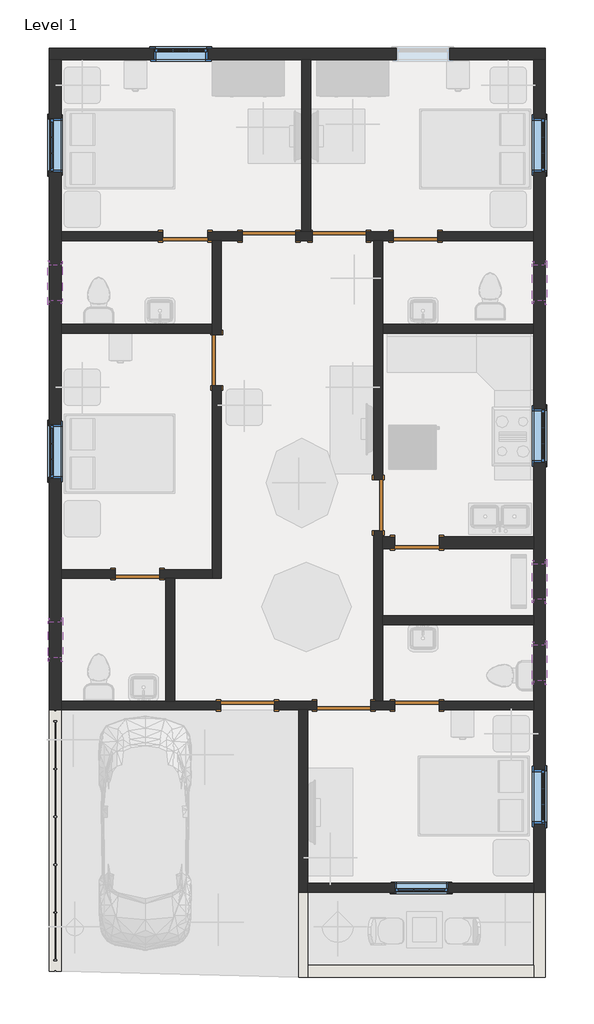
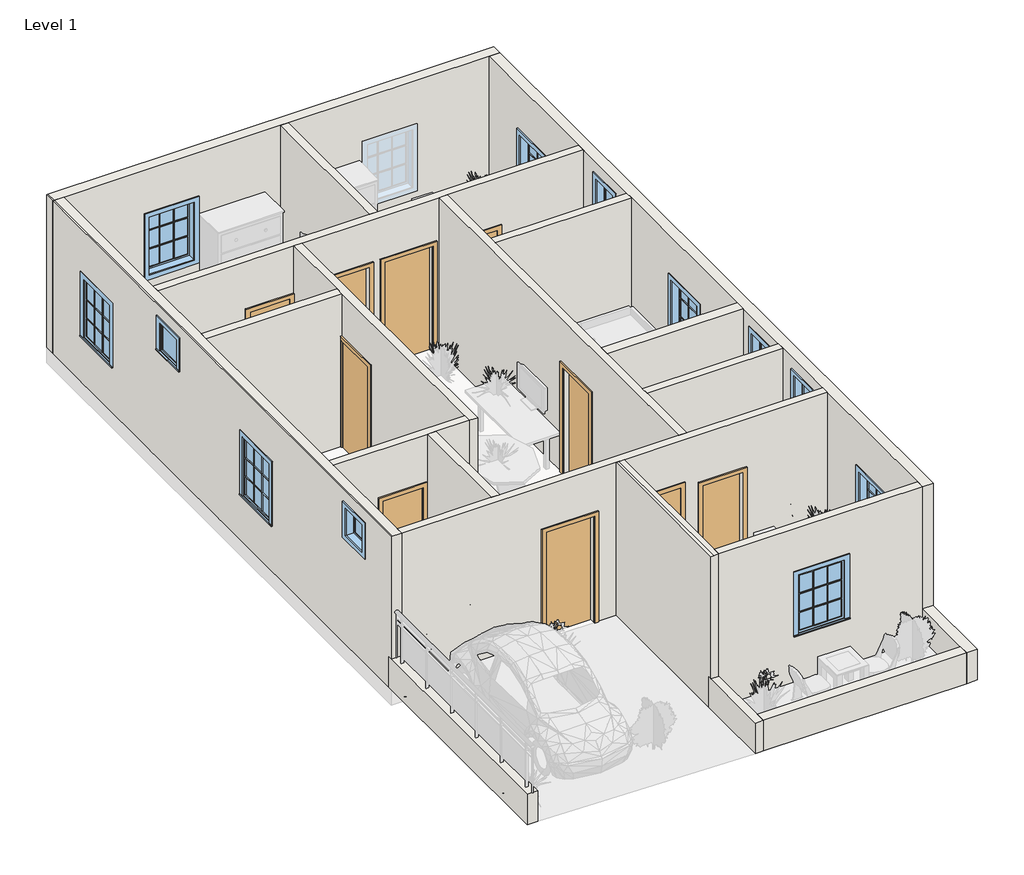
# One storey, part 1 of 2: 20 walls, 12 windows, 11 doors.
"""IFC4 building model written with IfcOpenShell, lengths in millimetres."""

from ifc_helpers import new_model, si_unit, frame, origin, origin_with_axes, place, context, project, spatial, polyline, outline, extrude, faceted_brep, transform, mapped, element, save
from components import door_255cab33, door_059fdd7e, door_fadea3f2, door_b6e9fca3, door_16372e1c, door_686f89d2, window_29c06734, window_5c190c7e, window_e41d21a6

model = new_model("IFC4")

# Units and contexts
model_context = context("Model", 3, world=origin())
ifc_project = project(units=[si_unit("LENGTHUNIT", "METRE", prefix="MILLI")], contexts=[model_context])

# Site, building, storey
site = spatial("IfcSite", under=ifc_project)
building = spatial("IfcBuilding", under=site)
storey = spatial("IfcBuildingStorey", under=building, Name="Level 1", Elevation=0.0)

# Doors
placement = place(None, origin())
door_shape = door_255cab33(model_context)
element("IfcDoor", 1, ObjectType="Single-Flush : 30\" x 80\"", at=placement, inside=storey, context=model_context, shape_type="MappedRepresentation", body=[
    mapped(door_shape, transform((-14104.3267032, 10209.9187882, 0.0), x_axis=(1.0, 0.0, 0.0), y_axis=(0.0, 1.0, 0.0), z_axis=(0.0, 0.0, 1.0))),
])
element("IfcDoor", 2, ObjectType="Single-Flush : 30\" x 80\"", at=placement, inside=storey, context=model_context, shape_type="MappedRepresentation", body=[
    mapped(door_shape, transform((-10167.3267032, 2234.3187882, 0.0), x_axis=(-1.0, 0.0, 0.0), y_axis=(0.0, -1.0, 0.0), z_axis=(0.0, 0.0, 1.0))),
])
element("IfcDoor", 3, ObjectType="Single-Flush : 30\" x 80\"", at=placement, inside=storey, context=model_context, shape_type="MappedRepresentation", body=[
    mapped(door_shape, transform((-14917.1267032, 4469.5187882, 0.0), x_axis=(1.0, 0.0, 0.0), y_axis=(0.0, 1.0, 0.0), z_axis=(0.0, 0.0, 1.0))),
])
door_2_shape = door_059fdd7e(model_context)
element("IfcDoor", 4, ObjectType="Single-Flush : 30\" x 80\"", at=placement, inside=storey, context=model_context, shape_type="MappedRepresentation", body=[
    mapped(door_2_shape, transform((-10192.7267032, 10209.9187882, 0.0), x_axis=(-1.0, 0.0, 0.0), y_axis=(0.0, -1.0, 0.0), z_axis=(0.0, 0.0, 1.0))),
])
door_3_shape = door_fadea3f2(model_context)
element("IfcDoor", 5, ObjectType="Single-Flush : 30\" x 80\"", at=placement, inside=storey, context=model_context, shape_type="MappedRepresentation", body=[
    mapped(door_3_shape, transform((-10167.3267032, 5002.9187882, 0.0), x_axis=(-1.0, 0.0, 0.0), y_axis=(0.0, -1.0, 0.0), z_axis=(0.0, 0.0, 1.0))),
])
door_4_shape = door_b6e9fca3(model_context)
element("IfcDoor", 6, ObjectType="Single-Flush : 34\" x 84\"", at=placement, inside=storey, context=model_context, shape_type="MappedRepresentation", body=[
    mapped(door_4_shape, transform((-13570.9267032, 8101.7187882, 0.0), x_axis=(0.0, 1.0, 0.0), y_axis=(-1.0, 0.0, 0.0), z_axis=(0.0, 0.0, 1.0))),
])
element("IfcDoor", 7, ObjectType="Single-Flush : 34\" x 84\"", at=placement, inside=storey, context=model_context, shape_type="MappedRepresentation", body=[
    mapped(door_4_shape, transform((-10827.7267032, 5637.9187882, 0.0), x_axis=(0.0, -1.0, 0.0), y_axis=(1.0, 0.0, 0.0), z_axis=(0.0, 0.0, 1.0))),
])
door_5_shape = door_16372e1c(model_context)
element("IfcDoor", 8, ObjectType="Single-Flush : 36\" x 84\"", at=placement, inside=storey, context=model_context, shape_type="MappedRepresentation", body=[
    mapped(door_5_shape, transform((-12681.9267032, 10209.9187882, 0.0), x_axis=(1.0, 0.0, 0.0), y_axis=(0.0, 1.0, 0.0), z_axis=(0.0, 0.0, 1.0))),
])
element("IfcDoor", 9, ObjectType="Single-Flush : 36\" x 84\"", at=placement, inside=storey, context=model_context, shape_type="MappedRepresentation", body=[
    mapped(door_5_shape, transform((-11411.9267032, 2234.3187882, 0.0), x_axis=(-1.0, 0.0, 0.0), y_axis=(0.0, -1.0, 0.0), z_axis=(0.0, 0.0, 1.0))),
])
door_6_shape = door_686f89d2(model_context)
element("IfcDoor", 10, ObjectType="Single-Flush : 36\" x 84\"", at=placement, inside=storey, context=model_context, shape_type="MappedRepresentation", body=[
    mapped(door_6_shape, transform((-11488.1267032, 10209.9187882, 0.0), x_axis=(-1.0, 0.0, 0.0), y_axis=(0.0, -1.0, 0.0), z_axis=(0.0, 0.0, 1.0))),
])
element("IfcDoor", 11, ObjectType="Single-Flush : 36\" x 84\"", at=placement, inside=storey, context=model_context, shape_type="MappedRepresentation", body=[
    mapped(door_6_shape, transform((-13050.2267032, 2234.3187882, 0.0), x_axis=(-1.0, 0.0, 0.0), y_axis=(0.0, -1.0, 0.0), z_axis=(0.0, 0.0, 1.0))),
])

# Walls
element("IfcWall", 12, ObjectType="Generic - 2'", at=placement, inside=storey, context=model_context, shape_type="Brep", body=[
    faceted_brep([(-16212.5267032, -2286.8812118, 0.0), (-16212.5267032, 2158.1187882, 0.0), (-16212.5267032, 2234.3187882, 0.0), (-16212.5267032, 2234.3187882, 609.6), (-16212.5267032, -2286.8812118, 609.6), (-16415.7267032, -2286.8812118, 0.0), (-16415.7267032, -2286.8812118, 609.6), (-16415.7267032, 2234.3187882, 609.6), (-16415.7267032, 2234.3187882, 0.0)], [[[0, 1, 2, 3, 4]], [[5, 6, 7, 8]], [[2, 1, 0, 5, 8]], [[3, 2, 8, 7]], [[4, 3, 7, 6]], [[0, 4, 6, 5]]]),
])
element("IfcWall", 13, ObjectType="Generic - 2'", at=placement, inside=storey, context=model_context, shape_type="SweptSolid", body=[
    extrude(outline(polyline([(-12021.5267032, -2185.2812118), (-8186.1267032, -2185.2812118), (-8186.1267032, -2388.4812118), (-12021.5267032, -2388.4812118), (-12021.5267032, -2185.2812118)])), origin_with_axes(), (0.0, 0.0, 1.0), 609.6),
])
element("IfcWall", 14, ObjectType="Generic - 2'", at=placement, inside=storey, context=model_context, shape_type="Brep", body=[
    faceted_brep([(-8186.1267032, -864.4812118, 0.0), (-8186.1267032, -940.6812118, 0.0), (-8186.1267032, -2185.2812118, 0.0), (-8186.1267032, -2388.4812118, 0.0), (-8186.1267032, -2388.4812118, 609.6), (-8186.1267032, -2185.2812118, 609.6), (-8186.1267032, -864.4812118, 609.6), (-7982.9267032, -864.4812118, 0.0), (-7982.9267032, -864.4812118, 609.6), (-7982.9267032, -2388.4812118, 609.6), (-7982.9267032, -2388.4812118, 0.0)], [[[0, 1, 2, 3, 4, 5, 6]], [[7, 8, 9, 10]], [[3, 2, 1, 0, 7, 10]], [[6, 5, 4, 9, 8]], [[0, 6, 8, 7]], [[4, 3, 10, 9]]]),
])
element("IfcWall", 15, ObjectType="Generic - 8\"", at=placement, inside=storey, context=model_context, shape_type="Brep", body=[
    faceted_brep([(-16415.7267032, 13207.1187882, 0.0), (-16212.5267032, 13207.1187882, 0.0), (-12123.1267032, 13207.1187882, 0.0), (-11970.7267032, 13207.1187882, 0.0), (-8186.1267032, 13207.1187882, 0.0), (-7982.9267032, 13207.1187882, 0.0), (-7982.9267032, 13207.1187882, 3048.0), (-8186.1267032, 13207.1187882, 3048.0), (-11970.7267032, 13207.1187882, 3048.0), (-12123.1267032, 13207.1187882, 3048.0), (-16212.5267032, 13207.1187882, 3048.0), (-16390.3267032, 13207.1187882, 3048.0), (-16415.7267032, 13207.1187882, 3048.0), (-13723.3267032, 13207.1187882, 2133.6), (-13723.3267032, 13207.1187882, 914.4), (-14637.7267032, 13207.1187882, 914.4), (-14637.7267032, 13207.1187882, 2133.6), (-9608.5267032, 13207.1187882, 2133.6), (-9608.5267032, 13207.1187882, 914.4), (-10522.9267032, 13207.1187882, 914.4), (-10522.9267032, 13207.1187882, 2133.6), (-16415.7267032, 13410.3187882, 0.0), (-16415.7267032, 13410.3187882, 3048.0), (-16390.3267032, 13410.3187882, 3048.0), (-7982.9267032, 13410.3187882, 3048.0), (-7982.9267032, 13410.3187882, 0.0), (-13723.3267032, 13410.3187882, 2133.6), (-14637.7267032, 13410.3187882, 2133.6), (-14637.7267032, 13410.3187882, 914.4), (-13723.3267032, 13410.3187882, 914.4), (-9608.5267032, 13410.3187882, 2133.6), (-10522.9267032, 13410.3187882, 2133.6), (-10522.9267032, 13410.3187882, 914.4), (-9608.5267032, 13410.3187882, 914.4)], [[[0, 1, 2, 3, 4, 5, 6, 7, 8, 9, 10, 11, 12], [13, 14, 15, 16], [17, 18, 19, 20]], [[21, 22, 23, 24, 25], [26, 27, 28, 29], [30, 31, 32, 33]], [[5, 4, 3, 2, 1, 0, 21, 25]], [[6, 5, 25, 24]], [[0, 12, 22, 21]], [[14, 13, 26, 29]], [[15, 14, 29, 28]], [[16, 15, 28, 27]], [[13, 16, 27, 26]], [[18, 17, 30, 33]], [[19, 18, 33, 32]], [[20, 19, 32, 31]], [[17, 20, 31, 30]], [[12, 11, 23, 22]], [[11, 10, 9, 8, 7, 6, 24, 23]]]),
])
element("IfcWall", 16, ObjectType="Generic - 8\"", at=placement, inside=storey, context=model_context, shape_type="Brep", body=[
    faceted_brep([(-8186.1267032, 13207.1187882, 0.0), (-8186.1267032, 10286.1187882, 0.0), (-8186.1267032, 10133.7187882, 0.0), (-8186.1267032, 8711.3187882, 0.0), (-8186.1267032, 8558.9187882, 0.0), (-8186.1267032, 5104.5187882, 0.0), (-8186.1267032, 4901.3187882, 0.0), (-8186.1267032, 3758.3187882, 0.0), (-8186.1267032, 3605.9187882, 0.0), (-8186.1267032, 2310.5187882, 0.0), (-8186.1267032, 2158.1187882, 0.0), (-8186.1267032, -788.2812118, 0.0), (-8186.1267032, -864.4812118, 0.0), (-8186.1267032, -864.4812118, 609.6), (-8186.1267032, -940.6812118, 609.6), (-8186.1267032, -940.6812118, 3048.0), (-8186.1267032, -788.2812118, 3048.0), (-8186.1267032, 2158.1187882, 3048.0), (-8186.1267032, 2310.5187882, 3048.0), (-8186.1267032, 3605.9187882, 3048.0), (-8186.1267032, 3758.3187882, 3048.0), (-8186.1267032, 4901.3187882, 3048.0), (-8186.1267032, 5104.5187882, 3048.0), (-8186.1267032, 8558.9187882, 3048.0), (-8186.1267032, 8711.3187882, 3048.0), (-8186.1267032, 10133.7187882, 3048.0), (-8186.1267032, 10286.1187882, 3048.0), (-8186.1267032, 13207.1187882, 3048.0), (-8186.1267032, 11302.1187882, 2133.6), (-8186.1267032, 11302.1187882, 914.4), (-8186.1267032, 12216.5187882, 914.4), (-8186.1267032, 12216.5187882, 2133.6), (-8186.1267032, 6361.8187882, 2235.2), (-8186.1267032, 6361.8187882, 1016.0), (-8186.1267032, 7276.2187882, 1016.0), (-8186.1267032, 7276.2187882, 2235.2), (-8186.1267032, 227.7187882, 2133.6), (-8186.1267032, 227.7187882, 914.4), (-8186.1267032, 1142.1187882, 914.4), (-8186.1267032, 1142.1187882, 2133.6), (-8186.1267032, 4037.7187882, 2768.6), (-8186.1267032, 4037.7187882, 2159.0), (-8186.1267032, 4647.3187882, 2159.0), (-8186.1267032, 4647.3187882, 2768.6), (-8186.1267032, 2653.4187882, 2768.6), (-8186.1267032, 2653.4187882, 2159.0), (-8186.1267032, 3263.0187882, 2159.0), (-8186.1267032, 3263.0187882, 2768.6), (-8186.1267032, 9117.7187882, 2768.6), (-8186.1267032, 9117.7187882, 2159.0), (-8186.1267032, 9727.3187882, 2159.0), (-8186.1267032, 9727.3187882, 2768.6), (-7982.9267032, 13207.1187882, 0.0), (-7982.9267032, 13207.1187882, 3048.0), (-7982.9267032, -940.6812118, 3048.0), (-7982.9267032, -940.6812118, 609.6), (-7982.9267032, -864.4812118, 609.6), (-7982.9267032, -864.4812118, 0.0), (-7982.9267032, 11302.1187882, 2133.6), (-7982.9267032, 12216.5187882, 2133.6), (-7982.9267032, 12216.5187882, 914.4), (-7982.9267032, 11302.1187882, 914.4), (-7982.9267032, 6361.8187882, 2235.2), (-7982.9267032, 7276.2187882, 2235.2), (-7982.9267032, 7276.2187882, 1016.0), (-7982.9267032, 6361.8187882, 1016.0), (-7982.9267032, 227.7187882, 2133.6), (-7982.9267032, 1142.1187882, 2133.6), (-7982.9267032, 1142.1187882, 914.4), (-7982.9267032, 227.7187882, 914.4), (-7982.9267032, 4037.7187882, 2768.6), (-7982.9267032, 4647.3187882, 2768.6), (-7982.9267032, 4647.3187882, 2159.0), (-7982.9267032, 4037.7187882, 2159.0), (-7982.9267032, 2653.4187882, 2768.6), (-7982.9267032, 3263.0187882, 2768.6), (-7982.9267032, 3263.0187882, 2159.0), (-7982.9267032, 2653.4187882, 2159.0), (-7982.9267032, 9117.7187882, 2768.6), (-7982.9267032, 9727.3187882, 2768.6), (-7982.9267032, 9727.3187882, 2159.0), (-7982.9267032, 9117.7187882, 2159.0)], [[[0, 1, 2, 3, 4, 5, 6, 7, 8, 9, 10, 11, 12, 13, 14, 15, 16, 17, 18, 19, 20, 21, 22, 23, 24, 25, 26, 27], [28, 29, 30, 31], [32, 33, 34, 35], [36, 37, 38, 39], [40, 41, 42, 43], [44, 45, 46, 47], [48, 49, 50, 51]], [[52, 53, 54, 55, 56, 57], [58, 59, 60, 61], [62, 63, 64, 65], [66, 67, 68, 69], [70, 71, 72, 73], [74, 75, 76, 77], [78, 79, 80, 81]], [[12, 11, 10, 9, 8, 7, 6, 5, 4, 3, 2, 1, 0, 52, 57]], [[0, 27, 53, 52]], [[29, 28, 58, 61]], [[30, 29, 61, 60]], [[31, 30, 60, 59]], [[28, 31, 59, 58]], [[33, 32, 62, 65]], [[34, 33, 65, 64]], [[35, 34, 64, 63]], [[32, 35, 63, 62]], [[37, 36, 66, 69]], [[38, 37, 69, 68]], [[39, 38, 68, 67]], [[36, 39, 67, 66]], [[41, 40, 70, 73]], [[42, 41, 73, 72]], [[43, 42, 72, 71]], [[40, 43, 71, 70]], [[45, 44, 74, 77]], [[46, 45, 77, 76]], [[47, 46, 76, 75]], [[44, 47, 75, 74]], [[49, 48, 78, 81]], [[50, 49, 81, 80]], [[51, 50, 80, 79]], [[48, 51, 79, 78]], [[13, 12, 57, 56]], [[55, 14, 13, 56]], [[15, 14, 55, 54]], [[27, 26, 25, 24, 23, 22, 21, 20, 19, 18, 17, 16, 15, 54, 53]]]),
])
element("IfcWall", 17, ObjectType="Generic - 8\"", at=placement, inside=storey, context=model_context, shape_type="SweptSolid", body=[
    extrude(outline(polyline([(0.0, -10751.5267032), (0.0, -10548.3267032), (2032.0, -10548.3267032), (2032.0, -9786.3267032), (0.0, -9786.3267032), (0.0, -8186.1267032), (3048.0, -8186.1267032), (3048.0, -10751.5267032), (0.0, -10751.5267032)])), frame((0.0, 4901.3187882, 0.0), z_axis=(0.0, 1.0, 0.0), x_axis=(0.0, 0.0, 1.0)), (0.0, 0.0, 1.0), 203.2),
])
element("IfcWall", 18, ObjectType="Generic - 8\"", at=placement, inside=storey, context=model_context, shape_type="Brep", body=[
    faceted_brep([(-16212.5267032, 2234.3187882, 0.0), (-16212.5267032, 2310.5187882, 0.0), (-16212.5267032, 4393.3187882, 0.0), (-16212.5267032, 4545.7187882, 0.0), (-16212.5267032, 8558.9187882, 0.0), (-16212.5267032, 8711.3187882, 0.0), (-16212.5267032, 10133.7187882, 0.0), (-16212.5267032, 10286.1187882, 0.0), (-16212.5267032, 13207.1187882, 0.0), (-16212.5267032, 13207.1187882, 3048.0), (-16212.5267032, 10286.1187882, 3048.0), (-16212.5267032, 10133.7187882, 3048.0), (-16212.5267032, 8711.3187882, 3048.0), (-16212.5267032, 8558.9187882, 3048.0), (-16212.5267032, 4545.7187882, 3048.0), (-16212.5267032, 4393.3187882, 3048.0), (-16212.5267032, 2310.5187882, 3048.0), (-16212.5267032, 2158.1187882, 3048.0), (-16212.5267032, 2158.1187882, 609.6), (-16212.5267032, 2234.3187882, 609.6), (-16212.5267032, 12216.5187882, 2133.6), (-16212.5267032, 12216.5187882, 914.4), (-16212.5267032, 11302.1187882, 914.4), (-16212.5267032, 11302.1187882, 2133.6), (-16212.5267032, 7009.5187882, 2133.6), (-16212.5267032, 7009.5187882, 914.4), (-16212.5267032, 6095.1187882, 914.4), (-16212.5267032, 6095.1187882, 2133.6), (-16212.5267032, 3047.1187882, 2768.6), (-16212.5267032, 3656.7187882, 2768.6), (-16212.5267032, 3656.7187882, 2159.0), (-16212.5267032, 3047.1187882, 2159.0), (-16212.5267032, 9727.3187882, 2768.6), (-16212.5267032, 9727.3187882, 2159.0), (-16212.5267032, 9117.7187882, 2159.0), (-16212.5267032, 9117.7187882, 2768.6), (-16415.7267032, 2234.3187882, 0.0), (-16415.7267032, 2234.3187882, 609.6), (-16415.7267032, 2158.1187882, 609.6), (-16415.7267032, 2158.1187882, 3048.0), (-16415.7267032, 13207.1187882, 3048.0), (-16415.7267032, 13207.1187882, 0.0), (-16415.7267032, 12216.5187882, 2133.6), (-16415.7267032, 11302.1187882, 2133.6), (-16415.7267032, 11302.1187882, 914.4), (-16415.7267032, 12216.5187882, 914.4), (-16415.7267032, 7009.5187882, 2133.6), (-16415.7267032, 6095.1187882, 2133.6), (-16415.7267032, 6095.1187882, 914.4), (-16415.7267032, 7009.5187882, 914.4), (-16415.7267032, 3047.1187882, 2768.6), (-16415.7267032, 3047.1187882, 2159.0), (-16415.7267032, 3656.7187882, 2159.0), (-16415.7267032, 3656.7187882, 2768.6), (-16415.7267032, 9727.3187882, 2768.6), (-16415.7267032, 9117.7187882, 2768.6), (-16415.7267032, 9117.7187882, 2159.0), (-16415.7267032, 9727.3187882, 2159.0), (-16390.3267032, 13207.1187882, 3048.0), (-16390.3267032, 2158.1187882, 3048.0)], [[[0, 1, 2, 3, 4, 5, 6, 7, 8, 9, 10, 11, 12, 13, 14, 15, 16, 17, 18, 19], [20, 21, 22, 23], [24, 25, 26, 27], [28, 29, 30, 31], [32, 33, 34, 35]], [[36, 37, 38, 39, 40, 41], [42, 43, 44, 45], [46, 47, 48, 49], [50, 51, 52, 53], [54, 55, 56, 57]], [[8, 7, 6, 5, 4, 3, 2, 1, 0, 36, 41]], [[9, 8, 41, 40, 58]], [[20, 23, 43, 42]], [[23, 22, 44, 43]], [[22, 21, 45, 44]], [[21, 20, 42, 45]], [[24, 27, 47, 46]], [[27, 26, 48, 47]], [[26, 25, 49, 48]], [[25, 24, 46, 49]], [[50, 53, 29, 28]], [[53, 52, 30, 29]], [[52, 51, 31, 30]], [[51, 50, 28, 31]], [[32, 35, 55, 54]], [[35, 34, 56, 55]], [[34, 33, 57, 56]], [[33, 32, 54, 57]], [[0, 19, 37, 36]], [[18, 38, 37, 19]], [[18, 17, 59, 39, 38]], [[58, 40, 39, 59]], [[17, 16, 15, 14, 13, 12, 11, 10, 9, 58, 59]]]),
])
element("IfcWall", 19, ObjectType="INNER 6\"", at=placement, inside=storey, context=model_context, shape_type="SweptSolid", body=[
    extrude(outline(polyline([(-12123.1267032, 10286.1187882), (-12123.1267032, 13207.1187882), (-11970.7267032, 13207.1187882), (-11970.7267032, 10286.1187882), (-12123.1267032, 10286.1187882)])), origin_with_axes(), (0.0, 0.0, 1.0), 3048.0),
])
element("IfcWall", 20, ObjectType="INNER 6\"", at=placement, inside=storey, context=model_context, shape_type="Brep", body=[
    faceted_brep([(-10573.7267032, 10286.1187882, 2032.0), (-10573.7267032, 10286.1187882, 0.0), (-11030.9267032, 10286.1187882, 0.0), (-11030.9267032, 10286.1187882, 2133.6), (-11945.3267032, 10286.1187882, 2133.6), (-11945.3267032, 10286.1187882, 0.0), (-11970.7267032, 10286.1187882, 0.0), (-12123.1267032, 10286.1187882, 0.0), (-12224.7267032, 10286.1187882, 0.0), (-12224.7267032, 10286.1187882, 2133.6), (-13139.1267032, 10286.1187882, 2133.6), (-13139.1267032, 10286.1187882, 0.0), (-13723.3267032, 10286.1187882, 0.0), (-13723.3267032, 10286.1187882, 2032.0), (-14485.3267032, 10286.1187882, 2032.0), (-14485.3267032, 10286.1187882, 0.0), (-16212.5267032, 10286.1187882, 0.0), (-16212.5267032, 10286.1187882, 3048.0), (-12123.1267032, 10286.1187882, 3048.0), (-11970.7267032, 10286.1187882, 3048.0), (-8186.1267032, 10286.1187882, 3048.0), (-8186.1267032, 10286.1187882, 0.0), (-9811.7267032, 10286.1187882, 0.0), (-9811.7267032, 10286.1187882, 2032.0), (-11030.9267032, 10133.7187882, 0.0), (-10903.9267032, 10133.7187882, 0.0), (-10751.5267032, 10133.7187882, 0.0), (-10573.7267032, 10133.7187882, 0.0), (-10573.7267032, 10133.7187882, 2032.0), (-9811.7267032, 10133.7187882, 2032.0), (-9811.7267032, 10133.7187882, 0.0), (-8186.1267032, 10133.7187882, 0.0), (-8186.1267032, 10133.7187882, 3048.0), (-10751.5267032, 10133.7187882, 3048.0), (-10903.9267032, 10133.7187882, 3048.0), (-13494.7267032, 10133.7187882, 3048.0), (-13647.1267032, 10133.7187882, 3048.0), (-16212.5267032, 10133.7187882, 3048.0), (-16212.5267032, 10133.7187882, 0.0), (-14485.3267032, 10133.7187882, 0.0), (-14485.3267032, 10133.7187882, 2032.0), (-13723.3267032, 10133.7187882, 2032.0), (-13723.3267032, 10133.7187882, 0.0), (-13647.1267032, 10133.7187882, 0.0), (-13494.7267032, 10133.7187882, 0.0), (-13139.1267032, 10133.7187882, 0.0), (-13139.1267032, 10133.7187882, 2133.6), (-12224.7267032, 10133.7187882, 2133.6), (-12224.7267032, 10133.7187882, 0.0), (-11945.3267032, 10133.7187882, 0.0), (-11945.3267032, 10133.7187882, 2133.6), (-11030.9267032, 10133.7187882, 2133.6)], [[[0, 1, 2, 3, 4, 5, 6, 7, 8, 9, 10, 11, 12, 13, 14, 15, 16, 17, 18, 19, 20, 21, 22, 23]], [[24, 25, 26, 27, 28, 29, 30, 31, 32, 33, 34, 35, 36, 37, 38, 39, 40, 41, 42, 43, 44, 45, 46, 47, 48, 49, 50, 51]], [[8, 7, 6, 5, 49, 48]], [[39, 38, 16, 15]], [[45, 44, 43, 42, 12, 11]], [[22, 21, 31, 30]], [[2, 1, 27, 26, 25, 24]], [[17, 16, 38, 37]], [[21, 20, 32, 31]], [[9, 8, 48, 47]], [[10, 9, 47, 46]], [[11, 10, 46, 45]], [[50, 49, 5, 4]], [[51, 50, 4, 3]], [[24, 51, 3, 2]], [[13, 12, 42, 41]], [[14, 13, 41, 40]], [[15, 14, 40, 39]], [[28, 27, 1, 0]], [[29, 28, 0, 23]], [[30, 29, 23, 22]], [[20, 19, 18, 17, 37, 36, 35, 34, 33, 32]]]),
])
element("IfcWall", 21, ObjectType="INNER 6\"", at=placement, inside=storey, context=model_context, shape_type="Brep", body=[
    faceted_brep([(-13647.1267032, 10133.7187882, 0.0), (-13647.1267032, 8711.3187882, 0.0), (-13647.1267032, 8558.9187882, 0.0), (-13647.1267032, 8533.5187882, 0.0), (-13647.1267032, 8533.5187882, 2133.6), (-13647.1267032, 7669.9187882, 2133.6), (-13647.1267032, 7669.9187882, 0.0), (-13647.1267032, 4545.7187882, 0.0), (-13647.1267032, 4393.3187882, 0.0), (-13647.1267032, 4393.3187882, 3048.0), (-13647.1267032, 4545.7187882, 3048.0), (-13647.1267032, 8558.9187882, 3048.0), (-13647.1267032, 8711.3187882, 3048.0), (-13647.1267032, 10133.7187882, 3048.0), (-13494.7267032, 8533.5187882, 2133.6), (-13494.7267032, 8533.5187882, 0.0), (-13494.7267032, 10133.7187882, 0.0), (-13494.7267032, 10133.7187882, 3048.0), (-13494.7267032, 4393.3187882, 3048.0), (-13494.7267032, 4393.3187882, 0.0), (-13494.7267032, 7669.9187882, 0.0), (-13494.7267032, 7669.9187882, 2133.6)], [[[0, 1, 2, 3, 4, 5, 6, 7, 8, 9, 10, 11, 12, 13]], [[14, 15, 16, 17, 18, 19, 20, 21]], [[20, 19, 8, 7, 6]], [[16, 15, 3, 2, 1, 0]], [[0, 13, 17, 16]], [[9, 8, 19, 18]], [[4, 3, 15, 14]], [[5, 4, 14, 21]], [[6, 5, 21, 20]], [[13, 12, 11, 10, 9, 18, 17]]]),
])
element("IfcWall", 22, ObjectType="INNER 6\"", at=placement, inside=storey, context=model_context, shape_type="SweptSolid", body=[
    extrude(outline(polyline([(-16212.5267032, 8711.3187882), (-13647.1267032, 8711.3187882), (-13647.1267032, 8558.9187882), (-16212.5267032, 8558.9187882), (-16212.5267032, 8711.3187882)])), origin_with_axes(), (0.0, 0.0, 1.0), 3048.0),
])
element("IfcWall", 23, ObjectType="INNER 6\"", at=placement, inside=storey, context=model_context, shape_type="SweptSolid", body=[
    extrude(outline(polyline([(-8186.1267032, 8558.9187882), (-10751.5267032, 8558.9187882), (-10751.5267032, 8711.3187882), (-8186.1267032, 8711.3187882), (-8186.1267032, 8558.9187882)])), origin_with_axes(), (0.0, 0.0, 1.0), 3048.0),
])
element("IfcWall", 24, ObjectType="INNER 6\"", at=placement, inside=storey, context=model_context, shape_type="Brep", body=[
    faceted_brep([(-10903.9267032, 5206.1187882, 2133.6), (-10903.9267032, 5206.1187882, 0.0), (-10903.9267032, 2310.5187882, 0.0), (-10903.9267032, 2310.5187882, 3048.0), (-10903.9267032, 10133.7187882, 3048.0), (-10903.9267032, 10133.7187882, 0.0), (-10903.9267032, 6069.7187882, 0.0), (-10903.9267032, 6069.7187882, 2133.6), (-10751.5267032, 2310.5187882, 0.0), (-10751.5267032, 3605.9187882, 0.0), (-10751.5267032, 3758.3187882, 0.0), (-10751.5267032, 4901.3187882, 0.0), (-10751.5267032, 5104.5187882, 0.0), (-10751.5267032, 5206.1187882, 0.0), (-10751.5267032, 5206.1187882, 2133.6), (-10751.5267032, 6069.7187882, 2133.6), (-10751.5267032, 6069.7187882, 0.0), (-10751.5267032, 8558.9187882, 0.0), (-10751.5267032, 8711.3187882, 0.0), (-10751.5267032, 10133.7187882, 0.0), (-10751.5267032, 10133.7187882, 3048.0), (-10751.5267032, 8711.3187882, 3048.0), (-10751.5267032, 8558.9187882, 3048.0), (-10751.5267032, 5104.5187882, 3048.0), (-10751.5267032, 4901.3187882, 3048.0), (-10751.5267032, 3758.3187882, 3048.0), (-10751.5267032, 3605.9187882, 3048.0), (-10751.5267032, 2310.5187882, 3048.0)], [[[0, 1, 2, 3, 4, 5, 6, 7]], [[8, 9, 10, 11, 12, 13, 14, 15, 16, 17, 18, 19, 20, 21, 22, 23, 24, 25, 26, 27]], [[6, 5, 19, 18, 17, 16]], [[2, 1, 13, 12, 11, 10, 9, 8]], [[5, 4, 20, 19]], [[3, 2, 8, 27]], [[14, 13, 1, 0]], [[15, 14, 0, 7]], [[16, 15, 7, 6]], [[4, 3, 27, 26, 25, 24, 23, 22, 21, 20]]]),
])
element("IfcWall", 25, ObjectType="INNER 6\"", at=placement, inside=storey, context=model_context, shape_type="Brep", body=[
    faceted_brep([(-13647.1267032, 4545.7187882, 0.0), (-14536.1267032, 4545.7187882, 0.0), (-14536.1267032, 4545.7187882, 2032.0), (-15298.1267032, 4545.7187882, 2032.0), (-15298.1267032, 4545.7187882, 0.0), (-16212.5267032, 4545.7187882, 0.0), (-16212.5267032, 4545.7187882, 3048.0), (-13647.1267032, 4545.7187882, 3048.0), (-14536.1267032, 4393.3187882, 2032.0), (-14536.1267032, 4393.3187882, 0.0), (-14434.5267032, 4393.3187882, 0.0), (-14282.1267032, 4393.3187882, 0.0), (-13647.1267032, 4393.3187882, 0.0), (-13647.1267032, 4393.3187882, 3048.0), (-14282.1267032, 4393.3187882, 3048.0), (-14434.5267032, 4393.3187882, 3048.0), (-16212.5267032, 4393.3187882, 3048.0), (-16212.5267032, 4393.3187882, 0.0), (-15298.1267032, 4393.3187882, 0.0), (-15298.1267032, 4393.3187882, 2032.0)], [[[0, 1, 2, 3, 4, 5, 6, 7]], [[8, 9, 10, 11, 12, 13, 14, 15, 16, 17, 18, 19]], [[18, 17, 5, 4]], [[12, 11, 10, 9, 1, 0]], [[0, 7, 13, 12]], [[6, 5, 17, 16]], [[2, 1, 9, 8]], [[3, 2, 8, 19]], [[4, 3, 19, 18]], [[7, 6, 16, 15, 14, 13]]]),
])
element("IfcWall", 26, ObjectType="INNER 6\"", at=placement, inside=storey, context=model_context, shape_type="SweptSolid", body=[
    extrude(outline(polyline([(-14434.5267032, 2310.5187882), (-14434.5267032, 4393.3187882), (-14282.1267032, 4393.3187882), (-14282.1267032, 2310.5187882), (-14434.5267032, 2310.5187882)])), origin_with_axes(), (0.0, 0.0, 1.0), 3048.0),
])
element("IfcWall", 27, ObjectType="INNER 6\"", at=placement, inside=storey, context=model_context, shape_type="Brep", body=[
    faceted_brep([(-16212.5267032, 2158.1187882, 0.0), (-13507.4267032, 2158.1187882, 0.0), (-13507.4267032, 2158.1187882, 2133.6), (-12593.0267032, 2158.1187882, 2133.6), (-12593.0267032, 2158.1187882, 0.0), (-12173.9267032, 2158.1187882, 0.0), (-12021.5267032, 2158.1187882, 0.0), (-11869.1267032, 2158.1187882, 0.0), (-11869.1267032, 2158.1187882, 2133.6), (-10954.7267032, 2158.1187882, 2133.6), (-10954.7267032, 2158.1187882, 0.0), (-10548.3267032, 2158.1187882, 0.0), (-10548.3267032, 2158.1187882, 2032.0), (-9786.3267032, 2158.1187882, 2032.0), (-9786.3267032, 2158.1187882, 0.0), (-8186.1267032, 2158.1187882, 0.0), (-8186.1267032, 2158.1187882, 3048.0), (-12021.5267032, 2158.1187882, 3048.0), (-12173.9267032, 2158.1187882, 3048.0), (-16212.5267032, 2158.1187882, 3048.0), (-16212.5267032, 2158.1187882, 609.6), (-13507.4267032, 2310.5187882, 2133.6), (-13507.4267032, 2310.5187882, 0.0), (-14282.1267032, 2310.5187882, 0.0), (-14434.5267032, 2310.5187882, 0.0), (-16212.5267032, 2310.5187882, 0.0), (-16212.5267032, 2310.5187882, 3048.0), (-14434.5267032, 2310.5187882, 3048.0), (-14282.1267032, 2310.5187882, 3048.0), (-10903.9267032, 2310.5187882, 3048.0), (-10751.5267032, 2310.5187882, 3048.0), (-8186.1267032, 2310.5187882, 3048.0), (-8186.1267032, 2310.5187882, 0.0), (-9786.3267032, 2310.5187882, 0.0), (-9786.3267032, 2310.5187882, 2032.0), (-10548.3267032, 2310.5187882, 2032.0), (-10548.3267032, 2310.5187882, 0.0), (-10751.5267032, 2310.5187882, 0.0), (-10903.9267032, 2310.5187882, 0.0), (-10954.7267032, 2310.5187882, 0.0), (-10954.7267032, 2310.5187882, 2133.6), (-11869.1267032, 2310.5187882, 2133.6), (-11869.1267032, 2310.5187882, 0.0), (-12593.0267032, 2310.5187882, 0.0), (-12593.0267032, 2310.5187882, 2133.6), (-16212.5267032, 2234.3187882, 0.0)], [[[0, 1, 2, 3, 4, 5, 6, 7, 8, 9, 10, 11, 12, 13, 14, 15, 16, 17, 18, 19, 20]], [[21, 22, 23, 24, 25, 26, 27, 28, 29, 30, 31, 32, 33, 34, 35, 36, 37, 38, 39, 40, 41, 42, 43, 44]], [[33, 32, 15, 14]], [[39, 38, 37, 36, 11, 10]], [[43, 42, 7, 6, 5, 4]], [[25, 24, 23, 22, 1, 0, 45]], [[16, 15, 32, 31]], [[12, 11, 36, 35]], [[13, 12, 35, 34]], [[14, 13, 34, 33]], [[8, 7, 42, 41]], [[9, 8, 41, 40]], [[10, 9, 40, 39]], [[2, 1, 22, 21]], [[3, 2, 21, 44]], [[4, 3, 44, 43]], [[19, 26, 25, 45, 0, 20]], [[19, 18, 17, 16, 31, 30, 29, 28, 27, 26]]]),
])
element("IfcWall", 28, ObjectType="INNER 6\"", at=placement, inside=storey, context=model_context, shape_type="Brep", body=[
    faceted_brep([(-12173.9267032, 2158.1187882, 0.0), (-12173.9267032, -864.4812118, 0.0), (-12173.9267032, -864.4812118, 609.6), (-12173.9267032, -940.6812118, 609.6), (-12173.9267032, -940.6812118, 3048.0), (-12173.9267032, 2158.1187882, 3048.0), (-12021.5267032, 2158.1187882, 0.0), (-12021.5267032, 2158.1187882, 3048.0), (-12021.5267032, -788.2812118, 3048.0), (-12021.5267032, -940.6812118, 3048.0), (-12021.5267032, -940.6812118, 609.6), (-12021.5267032, -864.4812118, 609.6), (-12021.5267032, -864.4812118, 0.0), (-12021.5267032, -788.2812118, 0.0), (-12123.1267032, 2158.1187882, 3048.0), (-12123.1267032, -940.6812118, 3048.0), (-12123.1267032, 2132.7187882, 3048.0)], [[[0, 1, 2, 3, 4, 5]], [[6, 7, 8, 9, 10, 11, 12, 13]], [[1, 0, 6, 13, 12]], [[0, 5, 14, 7, 6]], [[2, 1, 12, 11]], [[10, 3, 2, 11]], [[4, 3, 10, 9, 15]], [[5, 4, 15, 16, 14]], [[15, 9, 8, 7, 14, 16]]]),
])
element("IfcWall", 29, ObjectType="INNER 6\"", at=placement, inside=storey, context=model_context, shape_type="SweptSolid", body=[
    extrude(outline(polyline([(-8186.1267032, 3605.9187882), (-10751.5267032, 3605.9187882), (-10751.5267032, 3758.3187882), (-8186.1267032, 3758.3187882), (-8186.1267032, 3605.9187882)])), origin_with_axes(), (0.0, 0.0, 1.0), 3048.0),
])
element("IfcWall", 30, ObjectType="INNER 6\"", at=placement, inside=storey, context=model_context, shape_type="Brep", body=[
    faceted_brep([(-12021.5267032, -940.6812118, 3048.0), (-12021.5267032, -940.6812118, 609.6), (-12021.5267032, -940.6812118, 0.0), (-8186.1267032, -940.6812118, 0.0), (-8186.1267032, -940.6812118, 609.6), (-8186.1267032, -940.6812118, 3048.0), (-10548.3267032, -940.6812118, 2133.6), (-9633.9267032, -940.6812118, 2133.6), (-9633.9267032, -940.6812118, 914.4), (-10548.3267032, -940.6812118, 914.4), (-12021.5267032, -788.2812118, 0.0), (-12021.5267032, -788.2812118, 3048.0), (-8186.1267032, -788.2812118, 3048.0), (-8186.1267032, -788.2812118, 0.0), (-10548.3267032, -788.2812118, 2133.6), (-10548.3267032, -788.2812118, 914.4), (-9633.9267032, -788.2812118, 914.4), (-9633.9267032, -788.2812118, 2133.6), (-12021.5267032, -864.4812118, 0.0), (-8186.1267032, -864.4812118, 0.0)], [[[0, 1, 2, 3, 4, 5], [6, 7, 8, 9]], [[10, 11, 12, 13], [14, 15, 16, 17]], [[3, 2, 18, 10, 13, 19]], [[15, 14, 6, 9]], [[16, 15, 9, 8]], [[17, 16, 8, 7]], [[14, 17, 7, 6]], [[3, 19, 13, 12, 5, 4]], [[0, 11, 10, 18, 2, 1]], [[0, 5, 12, 11]]]),
])
element("IfcWall", 31, ObjectType="INNER 6\"", at=placement, inside=storey, context=model_context, shape_type="Brep", body=[
    faceted_brep([(-12173.9267032, -864.4812118, 0.0), (-12173.9267032, -2388.4812118, 0.0), (-12173.9267032, -2388.4812118, 609.6), (-12173.9267032, -940.6812118, 609.6), (-12173.9267032, -864.4812118, 609.6), (-12021.5267032, -864.4812118, 0.0), (-12021.5267032, -864.4812118, 609.6), (-12021.5267032, -940.6812118, 609.6), (-12021.5267032, -2185.2812118, 609.6), (-12021.5267032, -2388.4812118, 609.6), (-12021.5267032, -2388.4812118, 0.0), (-12021.5267032, -2185.2812118, 0.0), (-12021.5267032, -940.6812118, 0.0)], [[[0, 1, 2, 3, 4]], [[5, 6, 7, 8, 9, 10, 11, 12]], [[1, 0, 5, 12, 11, 10]], [[4, 3, 2, 9, 8, 7, 6]], [[0, 4, 6, 5]], [[2, 1, 10, 9]]]),
])

# Windows
window_shape = window_29c06734(model_context)
element("IfcWindow", 32, ObjectType="Casement 3x3 with Trim : 36\" x 48\"", at=placement, inside=storey, context=model_context, shape_type="MappedRepresentation", body=[
    mapped(window_shape, transform((-14180.5267032, 13308.7187882, 0.0), x_axis=(1.0, 0.0, 0.0), y_axis=(0.0, 1.0, 0.0), z_axis=(0.0, 0.0, 1.0))),
])
element("IfcWindow", 33, ObjectType="Casement 3x3 with Trim : 36\" x 48\"", at=placement, inside=storey, context=model_context, shape_type="MappedRepresentation", body=[
    mapped(window_shape, transform((-16314.1267032, 11759.3187882, 0.0), x_axis=(0.0, 1.0, 0.0), y_axis=(-1.0, 0.0, 0.0), z_axis=(0.0, 0.0, 1.0))),
])
element("IfcWindow", 34, ObjectType="Casement 3x3 with Trim : 36\" x 48\"", at=placement, inside=storey, context=model_context, shape_type="MappedRepresentation", body=[
    mapped(window_shape, transform((-16314.1267032, 6552.3187882, 0.0), x_axis=(0.0, 1.0, 0.0), y_axis=(-1.0, 0.0, 0.0), z_axis=(0.0, 0.0, 1.0))),
])
element("IfcWindow", 35, ObjectType="Casement 3x3 with Trim : 36\" x 48\"", at=placement, inside=storey, context=model_context, shape_type="MappedRepresentation", body=[
    mapped(window_shape, transform((-8084.5267032, 11759.3187882, 0.0), x_axis=(0.0, -1.0, 0.0), y_axis=(1.0, 0.0, 0.0), z_axis=(0.0, 0.0, 1.0))),
])
element("IfcWindow", 36, ObjectType="Casement 3x3 with Trim : 36\" x 48\"", at=placement, inside=storey, context=model_context, shape_type="MappedRepresentation", body=[
    mapped(window_shape, transform((-8084.5267032, 6819.0187882, 101.6), x_axis=(0.0, -1.0, 0.0), y_axis=(1.0, 0.0, 0.0), z_axis=(0.0, 0.0, 1.0))),
])
element("IfcWindow", 37, ObjectType="Casement 3x3 with Trim : 36\" x 48\"", at=placement, inside=storey, context=model_context, shape_type="MappedRepresentation", body=[
    mapped(window_shape, transform((-8084.5267032, 684.9187882, 0.0), x_axis=(0.0, -1.0, 0.0), y_axis=(1.0, 0.0, 0.0), z_axis=(0.0, 0.0, 1.0))),
])
window_2_shape = window_5c190c7e(model_context)
element("IfcWindow", 38, ObjectType="Casement 3x3 with Trim : 36\" x 48\"", at=placement, inside=storey, context=model_context, shape_type="MappedRepresentation", body=[
    mapped(window_2_shape, transform((-10091.1267032, -864.4812118, 0.0), x_axis=(-1.0, 0.0, 0.0), y_axis=(0.0, -1.0, 0.0), z_axis=(0.0, 0.0, 1.0))),
])
window_3_shape = window_e41d21a6(model_context)
element("IfcWindow", 39, ObjectType="Transom with Trim : 24\" x 24\"", at=placement, inside=storey, context=model_context, shape_type="MappedRepresentation", body=[
    mapped(window_3_shape, transform((-8084.5267032, 4304.4187882, 0.0), x_axis=(0.0, -1.0, 0.0), y_axis=(1.0, 0.0, 0.0), z_axis=(0.0, 0.0, 1.0))),
])
element("IfcWindow", 40, ObjectType="Transom with Trim : 24\" x 24\"", at=placement, inside=storey, context=model_context, shape_type="MappedRepresentation", body=[
    mapped(window_3_shape, transform((-8084.5267032, 2920.1187882, 0.0), x_axis=(0.0, -1.0, 0.0), y_axis=(1.0, 0.0, 0.0), z_axis=(0.0, 0.0, 1.0))),
])
element("IfcWindow", 41, ObjectType="Transom with Trim : 24\" x 24\"", at=placement, inside=storey, context=model_context, shape_type="MappedRepresentation", body=[
    mapped(window_3_shape, transform((-16314.1267032, 3313.8187882, 0.0), x_axis=(0.0, -1.0, 0.0), y_axis=(1.0, 0.0, 0.0), z_axis=(0.0, 0.0, 1.0))),
])
element("IfcWindow", 42, ObjectType="Transom with Trim : 24\" x 24\"", at=placement, inside=storey, context=model_context, shape_type="MappedRepresentation", body=[
    mapped(window_3_shape, transform((-16314.1267032, 9460.6187882, 0.0), x_axis=(0.0, 1.0, 0.0), y_axis=(-1.0, 0.0, 0.0), z_axis=(0.0, 0.0, 1.0))),
])
element("IfcWindow", 43, ObjectType="Transom with Trim : 24\" x 24\"", at=placement, inside=storey, context=model_context, shape_type="MappedRepresentation", body=[
    mapped(window_3_shape, transform((-8084.5267032, 9384.4187882, 0.0), x_axis=(0.0, -1.0, 0.0), y_axis=(1.0, 0.0, 0.0), z_axis=(0.0, 0.0, 1.0))),
])

save(model, "model.ifc")

# Revit data of these elements
# Type "Single-Flush : 30\" x 80\""
#   Type Mark = "5"
#   Construction Type Id = "MDOOR"
#   Assembly Code = "C1020"
#   Analytic Construction = "Metal"
#   Thickness = 0' - 2"
#   Heat Transfer Coefficient (U) = 0.651978 BTU/(h·ft²·°F)
#   Height = 6' - 8"
#   Trim Projection Ext = 0' - 1"
#   Trim Projection Int = 0' - 1"
#   Trim Width = 0' - 3"
#   Width = 2' - 6"
#   Define Thermal Properties by = 1
#   Door Material = Door - Panel
#   Frame Material = Door - Frame
#   Visual Light Transmittance = 0
#   Solar Heat Gain Coefficient = 0
#   Function = (empty or 0)
#   Wall Closure = (empty or 0)
# Type "Single-Flush : 34\" x 84\""
#   Type Mark = "2"
#   Construction Type Id = "MDOOR"
#   Assembly Code = "C1020"
#   Analytic Construction = "Metal"
#   Thickness = 0' - 2"
#   Heat Transfer Coefficient (U) = 0.651978 BTU/(h·ft²·°F)
#   Height = 7' - 0"
#   Trim Projection Ext = 0' - 1"
#   Trim Projection Int = 0' - 1"
#   Trim Width = 0' - 3"
#   Width = 2' - 10"
#   Define Thermal Properties by = 1
#   Door Material = Door - Panel
#   Frame Material = Door - Frame
#   Visual Light Transmittance = 0
#   Solar Heat Gain Coefficient = 0
#   Function = (empty or 0)
#   Wall Closure = (empty or 0)
# Type "Single-Flush : 36\" x 84\""
#   Type Mark = "1"
#   Construction Type Id = "MDOOR"
#   Assembly Code = "C1020"
#   Analytic Construction = "Metal"
#   Thickness = 0' - 2"
#   Heat Transfer Coefficient (U) = 0.651978 BTU/(h·ft²·°F)
#   Height = 7' - 0"
#   Trim Projection Ext = 0' - 1"
#   Trim Projection Int = 0' - 1"
#   Trim Width = 0' - 3"
#   Width = 3' - 0"
#   Define Thermal Properties by = 1
#   Door Material = Door - Panel
#   Frame Material = Door - Frame
#   Visual Light Transmittance = 0
#   Solar Heat Gain Coefficient = 0
#   Function = (empty or 0)
#   Wall Closure = (empty or 0)
# Type "Generic - 2'"
#   Assembly Code = "B2010"
#   Layers, outside or top first: 0' - 8" "Birch" (function 1)
# Type "Generic - 8\""
#   Assembly Code = "B2010"
#   Layers, outside or top first: 0' - 8" "Brick, Common" (function 1)
# Type "INNER 6\""
#   Assembly Code = "B2010"
#   Layers, outside or top first: 0' - 6" "Brick, Common" (function 1)
# Type "Casement 3x3 with Trim : 36\" x 48\""
#   Type Mark = "10"
#   Construction Type Id = "GSP4R"
#   Assembly Code = "B2020100"
#   Analytic Construction = "1/8 in Pilkington single glazing"
#   Visual Light Transmittance = 0.9
#   Solar Heat Gain Coefficient = 0.78
#   Heat Transfer Coefficient (U) = 0.6496 BTU/(h·ft²·°F)
#   Height = 4' - 0"
#   Default Sill Height = 3' - 0"
#   Trim Projection - Ext. = 0' - 0 1/2"
#   Trim Projection - Int. = 0' - 0 3/4"
#   Trim Width - Exterior = 0' - 3 1/2"
#   Trim Width - Interior = 0' - 3 1/2"
#   Width = 3' - 0"
#   Window Inset = 0' - 0 3/4"
#   Define Thermal Properties by = 1
#   Glass Pane Material = Glass
#   Sash Material = Sash
#   Trim Exterior Material = Trim
#   Trim Interior Material = Trim
#   Wall Closure = (empty or 0)
# Type "Transom with Trim : 24\" x 24\""
#   Type Mark = "13"
#   Construction Type Id = "GSP4R"
#   Assembly Code = "B2020100"
#   Analytic Construction = "1/8 in Pilkington single glazing"
#   Visual Light Transmittance = 0.9
#   Solar Heat Gain Coefficient = 0.78
#   Heat Transfer Coefficient (U) = 0.6496 BTU/(h·ft²·°F)
#   Height = 2' - 0"
#   Default Sill Height = 7' - 1"
#   Trim Projection - Ext. = 0' - 0 1/2"
#   Trim Projection - Int. = 0' - 0 3/4"
#   Trim Width - Exterior = 0' - 3 1/2"
#   Trim Width - Interior = 0' - 3 1/2"
#   Width = 2' - 0"
#   Window Inset = 0' - 0 3/4"
#   Define Thermal Properties by = 1
#   Glass Pane Material = Glass
#   Sash Material = Sash
#   Trim Exterior Material = Trim
#   Trim Interior Material = Trim
#   Wall Closure = (empty or 0)
# Elements 1, 2, 3, 4, 5 (IfcDoor, "Single-Flush : 30\" x 80\"")
#   Phase Created = New Construction
#   Materials on its faces: "Door - Frame", "Door - Panel"
# Elements 6, 7 (IfcDoor, "Single-Flush : 34\" x 84\"")
#   Phase Created = New Construction
#   Materials on its faces: "Door - Frame", "Door - Panel"
# Elements 8, 9, 10, 11 (IfcDoor, "Single-Flush : 36\" x 84\"")
#   Phase Created = New Construction
#   Materials on its faces: "Door - Frame", "Door - Panel"
# Elements 12, 13, 14 (IfcWall, "Generic - 2'")
#   Top Offset = 0' - 0"
#   Base Offset = 0' - 0"
#   Unconnected Height = 2' - 0"
#   wall height = 2' - 0"
#   Phase Created = New Construction
#   Base Constraint = Level 1
#   Materials on its faces: "Birch"
# Elements 15, 16, 17, 18 (IfcWall, "Generic - 8\"")
#   Top Offset = 0' - 0"
#   Base Offset = 0' - 0"
#   Unconnected Height = 10' - 0"
#   wall height = 10' - 0"
#   Phase Created = New Construction
#   Base Constraint = Level 1
#   Materials on its faces: "Brick, Common"
# Elements 19, 20, 21, 22, 23, 24, 25, 26, 27, 28, 29, 30 (IfcWall, "INNER 6\"")
#   Top Offset = 0' - 0"
#   Base Offset = 0' - 0"
#   Unconnected Height = 10' - 0"
#   wall height = 10' - 0"
#   Phase Created = New Construction
#   Base Constraint = Level 1
#   Materials on its faces: "Brick, Common"
# Element 31 (IfcWall, "INNER 6\"")
#   Top Offset = 0' - 0"
#   Base Offset = 0' - 0"
#   Unconnected Height = 2' - 0"
#   wall height = 2' - 0"
#   Phase Created = New Construction
#   Base Constraint = Level 1
#   Materials on its faces: "Brick, Common", "Birch"
# Element 32 (IfcWindow, "Casement 3x3 with Trim : 36\" x 48\"")
#   Mark = "1"
#   Phase Created = New Construction
#   Materials on its faces: "Sash", "Glass", "Trim"
# Element 33 (IfcWindow, "Casement 3x3 with Trim : 36\" x 48\"")
#   Mark = "2"
#   Phase Created = New Construction
#   Materials on its faces: "Sash", "Glass", "Trim"
# Element 34 (IfcWindow, "Casement 3x3 with Trim : 36\" x 48\"")
#   Mark = "3"
#   Phase Created = New Construction
#   Materials on its faces: "Sash", "Glass", "Trim"
# Element 35 (IfcWindow, "Casement 3x3 with Trim : 36\" x 48\"")
#   Mark = "6"
#   Phase Created = New Construction
#   Materials on its faces: "Sash", "Glass", "Trim"
# Element 36 (IfcWindow, "Casement 3x3 with Trim : 36\" x 48\"")
#   Mark = "7"
#   Phase Created = New Construction
#   Materials on its faces: "Sash", "Glass", "Trim"
# Element 37 (IfcWindow, "Casement 3x3 with Trim : 36\" x 48\"")
#   Mark = "8"
#   Phase Created = New Construction
#   Materials on its faces: "Sash", "Glass", "Trim"
# Element 38 (IfcWindow, "Casement 3x3 with Trim : 36\" x 48\"")
#   Mark = "9"
#   Phase Created = New Construction
#   Materials on its faces: "Sash", "Glass", "Trim"
# Element 39 (IfcWindow, "Transom with Trim : 24\" x 24\"")
#   Mark = "10"
#   Phase Created = New Construction
#   Materials on its faces: "Sash", "Trim", "Glass"
# Element 40 (IfcWindow, "Transom with Trim : 24\" x 24\"")
#   Mark = "11"
#   Phase Created = New Construction
#   Materials on its faces: "Sash", "Trim", "Glass"
# Element 41 (IfcWindow, "Transom with Trim : 24\" x 24\"")
#   Mark = "12"
#   Phase Created = New Construction
#   Materials on its faces: "Sash", "Trim", "Glass"
# Element 42 (IfcWindow, "Transom with Trim : 24\" x 24\"")
#   Mark = "13"
#   Phase Created = New Construction
#   Materials on its faces: "Sash", "Trim", "Glass"
# Element 43 (IfcWindow, "Transom with Trim : 24\" x 24\"")
#   Mark = "14"
#   Phase Created = New Construction
#   Materials on its faces: "Sash", "Trim", "Glass"
# Materials
#   "Door - Panel": class "Wood", colour RGB 210 159 95, transparency 0
#   "Door - Frame": colour RGB 118 70 51, transparency 0
#   "Birch": class "Wood", colour RGB 224 178 126, transparency 0, Description = "Betula Alleghaniensis", Cost = 0
#   "Brick, Common": class "Masonry", colour RGB 170 98 104, transparency 0, Description = "Common brick", Cost = 0
#   "Glass": class "Glass", colour RGB 0 128 192, transparency 0.75, Description = "Soda Lime Glass", Cost = 0
#   "Sash": class "Wood", colour RGB 224 178 126, transparency 0
#   "Trim": class "Wood", colour RGB 224 178 126, transparency 0
# Room at (-9651.278, 6611.577) mm, phase "New Construction", upper level "Level 1", upper offset 10' - 0", lower offset 0' - 0"
#   Number = "9"
#   Name = "KITCHEN"
# Room at (-15078.961, 9106.163) mm, phase "New Construction", upper level "Level 1", upper offset 10' - 0", lower offset 0' - 0"
#   Number = "2"
# Room at (-9651.278, 9325.248) mm, phase "New Construction", upper level "Level 1", upper offset 10' - 0", lower offset 0' - 0"
#   Number = "3"
# Room at (-10119.191, -1603.091) mm, phase "New Construction", upper level "Level 1", upper offset 10' - 0", lower offset 0' - 0"
#   Number = "10"
#   Name = "BALCONY"
# Room at (-12861.941, -1031.026) mm, phase "New Construction", upper level "Level 1", upper offset 10' - 0", lower offset 0' - 0"
#   Number = "11"
#   Name = "PORCH"
# Room at (-14682.887, 6230.671) mm, phase "New Construction", upper level "Level 1", upper offset 10' - 0", lower offset 0' - 0"
#   Number = "4"
#   Name = "GUEST ROOM"
# Room at (-15414.786, 3396.646) mm, phase "New Construction", upper level "Level 1", upper offset 10' - 0", lower offset 0' - 0"
#   Number = "5"
#   Name = "TOILET"
# Room at (-14506.375, 11743.673) mm, phase "New Construction", upper level "Level 1", upper offset 10' - 0", lower offset 0' - 0"
#   Number = "1"
#   Name = "BEDROOM"
# Room at (-10296.247, 535.93) mm, phase "New Construction", upper level "Level 1", upper offset 10' - 0", lower offset 0' - 0"
#   Number = "6"
#   Name = "MASTER BEDROOM"
# Room at (-9280.779, 2789) mm, phase "New Construction", upper level "Level 1", upper offset 10' - 0", lower offset 0' - 0"
#   Number = "7"
#   Name = "TOILET"
# Room at (-9652.112, 4248.736) mm, phase "New Construction", upper level "Level 1", upper offset 10' - 0", lower offset 0' - 0"
#   Number = "8"
#   Name = "STORE"
